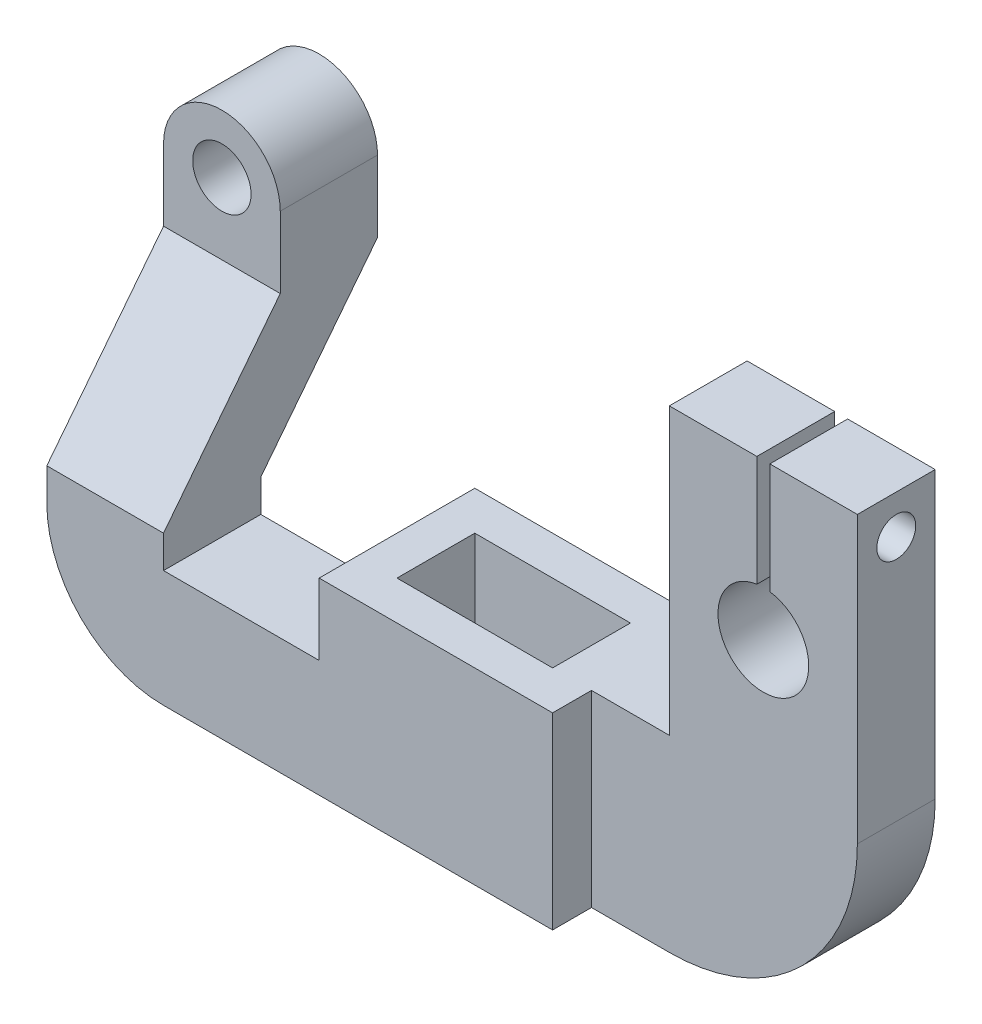
ISO-10303-21;
HEADER;
FILE_DESCRIPTION(('STEP AP214'),'2;1');
FILE_NAME('part.step','',(''),(''),'','','');
FILE_SCHEMA(('AUTOMOTIVE_DESIGN { 1 0 10303 214 1 1 1 1 }'));
ENDSEC;
DATA;
#1=APPLICATION_CONTEXT('core data for automotive mechanical design processes');
#2=APPLICATION_PROTOCOL_DEFINITION('international standard','automotive_design',2000,#1);
#3=PRODUCT_CONTEXT('',#1,'mechanical');
#4=PRODUCT('Part','Part','',(#3));
#5=PRODUCT_RELATED_PRODUCT_CATEGORY('part','',(#4));
#6=PRODUCT_DEFINITION_FORMATION('','',#4);
#7=PRODUCT_DEFINITION_CONTEXT('part definition',#1,'design');
#8=PRODUCT_DEFINITION('design','',#6,#7);
#9=PRODUCT_DEFINITION_SHAPE('','',#8);
#10=(LENGTH_UNIT() NAMED_UNIT(*) SI_UNIT(.MILLI.,.METRE.));
#11=(NAMED_UNIT(*) PLANE_ANGLE_UNIT() SI_UNIT($,.RADIAN.));
#12=(NAMED_UNIT(*) SI_UNIT($,.STERADIAN.) SOLID_ANGLE_UNIT());
#13=UNCERTAINTY_MEASURE_WITH_UNIT(LENGTH_MEASURE(1.E-05),#10,'distance_accuracy_value','');
#14=(GEOMETRIC_REPRESENTATION_CONTEXT(3) GLOBAL_UNCERTAINTY_ASSIGNED_CONTEXT((#13)) GLOBAL_UNIT_ASSIGNED_CONTEXT((#10,
#11,#12)) REPRESENTATION_CONTEXT('',''));
#15=CARTESIAN_POINT('',(0.,0.,0.));
#16=DIRECTION('',(0.,0.,1.));
#17=DIRECTION('',(1.,0.,0.));
#18=AXIS2_PLACEMENT_3D('',#15,#16,#17);
#19=CARTESIAN_POINT('',(48.,44.,6.));
#20=DIRECTION('',(0.,1.,0.));
#21=DIRECTION('',(0.,0.,1.));
#22=AXIS2_PLACEMENT_3D('',#19,#20,#21);
#23=PLANE('',#22);
#24=DIRECTION('',(0.,0.,1.));
#25=VECTOR('',#24,1.);
#26=CARTESIAN_POINT('',(63.5,44.,6.));
#27=LINE('',#26,#25);
#28=CARTESIAN_POINT('',(63.5,44.,6.));
#29=VERTEX_POINT('',#28);
#30=CARTESIAN_POINT('',(63.5,44.,18.));
#31=VERTEX_POINT('',#30);
#32=EDGE_CURVE('E285',#29,#31,#27,.T.);
#33=ORIENTED_EDGE('',*,*,#32,.T.);
#34=DIRECTION('',(-1.,0.,0.));
#35=VECTOR('',#34,1.);
#36=CARTESIAN_POINT('',(48.,44.,18.));
#37=LINE('',#36,#35);
#38=CARTESIAN_POINT('',(77.,44.,18.));
#39=VERTEX_POINT('',#38);
#40=EDGE_CURVE('E307',#39,#31,#37,.T.);
#41=ORIENTED_EDGE('',*,*,#40,.F.);
#42=DIRECTION('',(0.,0.,1.));
#43=VECTOR('',#42,1.);
#44=CARTESIAN_POINT('',(77.,44.,6.));
#45=LINE('',#44,#43);
#46=CARTESIAN_POINT('',(77.,44.,6.));
#47=VERTEX_POINT('',#46);
#48=EDGE_CURVE('E304',#47,#39,#45,.T.);
#49=ORIENTED_EDGE('',*,*,#48,.F.);
#50=DIRECTION('',(-1.,0.,0.));
#51=VECTOR('',#50,1.);
#52=CARTESIAN_POINT('',(48.,44.,6.));
#53=LINE('',#52,#51);
#54=EDGE_CURVE('E299',#47,#29,#53,.T.);
#55=ORIENTED_EDGE('',*,*,#54,.T.);
#56=EDGE_LOOP('',(#33,#41,#49,#55));
#57=FACE_BOUND('',#56,.T.);
#58=ADVANCED_FACE('F50',(#57),#23,.T.);
#59=CARTESIAN_POINT('',(0.,0.,24.));
#60=DIRECTION('',(0.,-1.,0.));
#61=DIRECTION('',(0.,0.,-1.));
#62=AXIS2_PLACEMENT_3D('',#59,#60,#61);
#63=PLANE('',#62);
#64=DIRECTION('',(1.,0.,0.));
#65=VECTOR('',#64,1.);
#66=CARTESIAN_POINT('',(6.,0.,18.));
#67=LINE('',#66,#65);
#68=CARTESIAN_POINT('',(6.,0.,18.));
#69=VERTEX_POINT('',#68);
#70=CARTESIAN_POINT('',(30.,0.,18.));
#71=VERTEX_POINT('',#70);
#72=EDGE_CURVE('E252',#69,#71,#67,.T.);
#73=ORIENTED_EDGE('',*,*,#72,.F.);
#74=DIRECTION('',(0.,0.,1.));
#75=VECTOR('',#74,1.);
#76=CARTESIAN_POINT('',(6.,0.,6.));
#77=LINE('',#76,#75);
#78=CARTESIAN_POINT('',(6.,0.,6.));
#79=VERTEX_POINT('',#78);
#80=EDGE_CURVE('E65',#79,#69,#77,.T.);
#81=ORIENTED_EDGE('',*,*,#80,.F.);
#82=DIRECTION('',(-1.,0.,0.));
#83=VECTOR('',#82,1.);
#84=CARTESIAN_POINT('',(6.,0.,6.));
#85=LINE('',#84,#83);
#86=CARTESIAN_POINT('',(30.,0.,6.));
#87=VERTEX_POINT('',#86);
#88=EDGE_CURVE('E260',#87,#79,#85,.T.);
#89=ORIENTED_EDGE('',*,*,#88,.F.);
#90=DIRECTION('',(0.,0.,-1.));
#91=VECTOR('',#90,1.);
#92=CARTESIAN_POINT('',(30.,0.,6.));
#93=LINE('',#92,#91);
#94=EDGE_CURVE('E245',#71,#87,#93,.T.);
#95=ORIENTED_EDGE('',*,*,#94,.F.);
#96=EDGE_LOOP('',(#73,#81,#89,#95));
#97=FACE_BOUND('',#96,.T.);
#98=DIRECTION('',(0.,0.,1.));
#99=VECTOR('',#98,1.);
#100=CARTESIAN_POINT('',(48.,0.,6.));
#101=LINE('',#100,#99);
#102=CARTESIAN_POINT('',(48.,0.,6.));
#103=VERTEX_POINT('',#102);
#104=CARTESIAN_POINT('',(48.,0.,18.));
#105=VERTEX_POINT('',#104);
#106=EDGE_CURVE('E313',#103,#105,#101,.T.);
#107=ORIENTED_EDGE('',*,*,#106,.F.);
#108=DIRECTION('',(-1.,0.,0.));
#109=VECTOR('',#108,1.);
#110=CARTESIAN_POINT('',(0.,0.,6.));
#111=LINE('',#110,#109);
#112=CARTESIAN_POINT('',(36.,0.,6.));
#113=VERTEX_POINT('',#112);
#114=EDGE_CURVE('E329',#103,#113,#111,.T.);
#115=ORIENTED_EDGE('',*,*,#114,.T.);
#116=DIRECTION('',(0.,0.,-1.));
#117=VECTOR('',#116,1.);
#118=CARTESIAN_POINT('',(36.,0.,24.));
#119=LINE('',#118,#117);
#120=CARTESIAN_POINT('',(36.,0.,0.));
#121=VERTEX_POINT('',#120);
#122=EDGE_CURVE('E457',#113,#121,#119,.T.);
#123=ORIENTED_EDGE('',*,*,#122,.T.);
#124=DIRECTION('',(-1.,0.,0.));
#125=VECTOR('',#124,1.);
#126=CARTESIAN_POINT('',(0.,0.,0.));
#127=LINE('',#126,#125);
#128=CARTESIAN_POINT('',(0.,0.,0.));
#129=VERTEX_POINT('',#128);
#130=EDGE_CURVE('E437',#121,#129,#127,.T.);
#131=ORIENTED_EDGE('',*,*,#130,.T.);
#132=DIRECTION('',(0.,0.,-1.));
#133=VECTOR('',#132,1.);
#134=CARTESIAN_POINT('',(0.,0.,24.));
#135=LINE('',#134,#133);
#136=CARTESIAN_POINT('',(0.,0.,24.));
#137=VERTEX_POINT('',#136);
#138=EDGE_CURVE('E444',#137,#129,#135,.T.);
#139=ORIENTED_EDGE('',*,*,#138,.F.);
#140=DIRECTION('',(-1.,0.,0.));
#141=VECTOR('',#140,1.);
#142=CARTESIAN_POINT('',(0.,0.,24.));
#143=LINE('',#142,#141);
#144=CARTESIAN_POINT('',(36.,0.,24.));
#145=VERTEX_POINT('',#144);
#146=EDGE_CURVE('E442',#145,#137,#143,.T.);
#147=ORIENTED_EDGE('',*,*,#146,.F.);
#148=CARTESIAN_POINT('',(36.,0.,18.));
#149=VERTEX_POINT('',#148);
#150=EDGE_CURVE('E459',#145,#149,#119,.T.);
#151=ORIENTED_EDGE('',*,*,#150,.T.);
#152=DIRECTION('',(1.,0.,0.));
#153=VECTOR('',#152,1.);
#154=CARTESIAN_POINT('',(0.,0.,18.));
#155=LINE('',#154,#153);
#156=EDGE_CURVE('E331',#149,#105,#155,.T.);
#157=ORIENTED_EDGE('',*,*,#156,.T.);
#158=EDGE_LOOP('',(#107,#115,#123,#131,#139,#147,#151,#157));
#159=FACE_BOUND('',#158,.T.);
#160=ADVANCED_FACE('F253',(#97,#159),#63,.F.);
#161=CARTESIAN_POINT('',(36.,0.,24.));
#162=DIRECTION('',(-1.,0.,0.));
#163=DIRECTION('',(0.,0.,1.));
#164=AXIS2_PLACEMENT_3D('',#161,#162,#163);
#165=PLANE('',#164);
#166=DIRECTION('',(0.,1.,0.));
#167=VECTOR('',#166,1.);
#168=CARTESIAN_POINT('',(36.,-29.,6.));
#169=LINE('',#168,#167);
#170=CARTESIAN_POINT('',(36.,-29.,6.));
#171=VERTEX_POINT('',#170);
#172=EDGE_CURVE('E336',#171,#113,#169,.T.);
#173=ORIENTED_EDGE('',*,*,#172,.F.);
#174=DIRECTION('',(0.,0.,-1.));
#175=VECTOR('',#174,1.);
#176=CARTESIAN_POINT('',(36.,-29.,24.));
#177=LINE('',#176,#175);
#178=CARTESIAN_POINT('',(36.,-29.,0.));
#179=VERTEX_POINT('',#178);
#180=EDGE_CURVE('E463',#171,#179,#177,.T.);
#181=ORIENTED_EDGE('',*,*,#180,.T.);
#182=DIRECTION('',(0.,1.,0.));
#183=VECTOR('',#182,1.);
#184=CARTESIAN_POINT('',(36.,0.,0.));
#185=LINE('',#184,#183);
#186=EDGE_CURVE('E454',#179,#121,#185,.T.);
#187=ORIENTED_EDGE('',*,*,#186,.T.);
#188=ORIENTED_EDGE('',*,*,#122,.F.);
#189=EDGE_LOOP('',(#173,#181,#187,#188));
#190=FACE_BOUND('',#189,.T.);
#191=ADVANCED_FACE('F499',(#190),#165,.F.);
#192=CARTESIAN_POINT('',(0.,-29.,24.));
#193=DIRECTION('',(1.,0.,0.));
#194=DIRECTION('',(0.,0.,-1.));
#195=AXIS2_PLACEMENT_3D('',#192,#193,#194);
#196=PLANE('',#195);
#197=DIRECTION('',(0.,0.,-1.));
#198=VECTOR('',#197,1.);
#199=CARTESIAN_POINT('',(0.,-29.,24.));
#200=LINE('',#199,#198);
#201=CARTESIAN_POINT('',(0.,-29.,9.));
#202=VERTEX_POINT('',#201);
#203=CARTESIAN_POINT('',(0.,-29.,0.));
#204=VERTEX_POINT('',#203);
#205=EDGE_CURVE('E462',#202,#204,#200,.T.);
#206=ORIENTED_EDGE('',*,*,#205,.F.);
#207=DIRECTION('',(0.,1.,0.));
#208=VECTOR('',#207,1.);
#209=CARTESIAN_POINT('',(0.,-11.,9.));
#210=LINE('',#209,#208);
#211=CARTESIAN_POINT('',(0.,-11.,9.));
#212=VERTEX_POINT('',#211);
#213=EDGE_CURVE('E387',#202,#212,#210,.T.);
#214=ORIENTED_EDGE('',*,*,#213,.T.);
#215=DIRECTION('',(0.,0.,1.));
#216=VECTOR('',#215,1.);
#217=CARTESIAN_POINT('',(0.,-11.,9.));
#218=LINE('',#217,#216);
#219=CARTESIAN_POINT('',(0.,-11.,24.));
#220=VERTEX_POINT('',#219);
#221=EDGE_CURVE('E412',#212,#220,#218,.T.);
#222=ORIENTED_EDGE('',*,*,#221,.T.);
#223=DIRECTION('',(0.,-1.,0.));
#224=VECTOR('',#223,1.);
#225=CARTESIAN_POINT('',(0.,-29.,24.));
#226=LINE('',#225,#224);
#227=EDGE_CURVE('E434',#137,#220,#226,.T.);
#228=ORIENTED_EDGE('',*,*,#227,.F.);
#229=ORIENTED_EDGE('',*,*,#138,.T.);
#230=DIRECTION('',(0.,-1.,0.));
#231=VECTOR('',#230,1.);
#232=CARTESIAN_POINT('',(0.,-29.,0.));
#233=LINE('',#232,#231);
#234=EDGE_CURVE('E426',#129,#204,#233,.T.);
#235=ORIENTED_EDGE('',*,*,#234,.T.);
#236=EDGE_LOOP('',(#206,#214,#222,#228,#229,#235));
#237=FACE_BOUND('',#236,.T.);
#238=ADVANCED_FACE('F47',(#237),#196,.F.);
#239=CARTESIAN_POINT('',(36.,-29.,24.));
#240=DIRECTION('',(0.,1.,0.));
#241=DIRECTION('',(0.,0.,1.));
#242=AXIS2_PLACEMENT_3D('',#239,#240,#241);
#243=PLANE('',#242);
#244=DIRECTION('',(-1.,0.,0.));
#245=VECTOR('',#244,1.);
#246=CARTESIAN_POINT('',(36.,-29.,6.));
#247=LINE('',#246,#245);
#248=CARTESIAN_POINT('',(30.,-29.,6.));
#249=VERTEX_POINT('',#248);
#250=CARTESIAN_POINT('',(6.,-29.,6.));
#251=VERTEX_POINT('',#250);
#252=EDGE_CURVE('E57',#249,#251,#247,.T.);
#253=ORIENTED_EDGE('',*,*,#252,.T.);
#254=DIRECTION('',(0.,0.,1.));
#255=VECTOR('',#254,1.);
#256=CARTESIAN_POINT('',(6.,-29.,24.));
#257=LINE('',#256,#255);
#258=CARTESIAN_POINT('',(6.,-29.,18.));
#259=VERTEX_POINT('',#258);
#260=EDGE_CURVE('E11',#251,#259,#257,.T.);
#261=ORIENTED_EDGE('',*,*,#260,.T.);
#262=DIRECTION('',(1.,0.,0.));
#263=VECTOR('',#262,1.);
#264=CARTESIAN_POINT('',(36.,-29.,18.));
#265=LINE('',#264,#263);
#266=CARTESIAN_POINT('',(30.,-29.,18.));
#267=VERTEX_POINT('',#266);
#268=EDGE_CURVE('E470',#259,#267,#265,.T.);
#269=ORIENTED_EDGE('',*,*,#268,.T.);
#270=DIRECTION('',(0.,0.,-1.));
#271=VECTOR('',#270,1.);
#272=CARTESIAN_POINT('',(30.,-29.,24.));
#273=LINE('',#272,#271);
#274=EDGE_CURVE('E244',#267,#249,#273,.T.);
#275=ORIENTED_EDGE('',*,*,#274,.T.);
#276=EDGE_LOOP('',(#253,#261,#269,#275));
#277=FACE_BOUND('',#276,.T.);
#278=DIRECTION('',(1.,0.,0.));
#279=VECTOR('',#278,1.);
#280=CARTESIAN_POINT('',(36.,-29.,0.));
#281=LINE('',#280,#279);
#282=EDGE_CURVE('E449',#204,#179,#281,.T.);
#283=ORIENTED_EDGE('',*,*,#282,.T.);
#284=ORIENTED_EDGE('',*,*,#180,.F.);
#285=DIRECTION('',(-1.,0.,0.));
#286=VECTOR('',#285,1.);
#287=CARTESIAN_POINT('',(0.,-29.,6.));
#288=LINE('',#287,#286);
#289=CARTESIAN_POINT('',(48.,-29.,6.));
#290=VERTEX_POINT('',#289);
#291=EDGE_CURVE('E335',#290,#171,#288,.T.);
#292=ORIENTED_EDGE('',*,*,#291,.F.);
#293=DIRECTION('',(0.,0.,-1.));
#294=VECTOR('',#293,1.);
#295=CARTESIAN_POINT('',(48.,-29.,0.));
#296=LINE('',#295,#294);
#297=CARTESIAN_POINT('',(48.,-29.,18.));
#298=VERTEX_POINT('',#297);
#299=EDGE_CURVE('E328',#298,#290,#296,.T.);
#300=ORIENTED_EDGE('',*,*,#299,.F.);
#301=DIRECTION('',(1.,0.,0.));
#302=VECTOR('',#301,1.);
#303=CARTESIAN_POINT('',(0.,-29.,18.));
#304=LINE('',#303,#302);
#305=CARTESIAN_POINT('',(36.,-29.,18.));
#306=VERTEX_POINT('',#305);
#307=EDGE_CURVE('E332',#306,#298,#304,.T.);
#308=ORIENTED_EDGE('',*,*,#307,.F.);
#309=CARTESIAN_POINT('',(36.,-29.,24.));
#310=VERTEX_POINT('',#309);
#311=EDGE_CURVE('E465',#310,#306,#177,.T.);
#312=ORIENTED_EDGE('',*,*,#311,.F.);
#313=DIRECTION('',(1.,0.,0.));
#314=VECTOR('',#313,1.);
#315=CARTESIAN_POINT('',(36.,-29.,24.));
#316=LINE('',#315,#314);
#317=CARTESIAN_POINT('',(-24.,-29.,24.));
#318=VERTEX_POINT('',#317);
#319=EDGE_CURVE('E438',#318,#310,#316,.T.);
#320=ORIENTED_EDGE('',*,*,#319,.F.);
#321=DIRECTION('',(0.,0.,1.));
#322=VECTOR('',#321,1.);
#323=CARTESIAN_POINT('',(-24.,-29.,9.));
#324=LINE('',#323,#322);
#325=CARTESIAN_POINT('',(-24.,-29.,9.));
#326=VERTEX_POINT('',#325);
#327=EDGE_CURVE('E424',#326,#318,#324,.T.);
#328=ORIENTED_EDGE('',*,*,#327,.F.);
#329=DIRECTION('',(1.,0.,0.));
#330=VECTOR('',#329,1.);
#331=CARTESIAN_POINT('',(0.,-29.,9.));
#332=LINE('',#331,#330);
#333=EDGE_CURVE('E408',#326,#202,#332,.T.);
#334=ORIENTED_EDGE('',*,*,#333,.T.);
#335=ORIENTED_EDGE('',*,*,#205,.T.);
#336=EDGE_LOOP('',(#283,#284,#292,#300,#308,#312,#320,#328,#334,#335));
#337=FACE_BOUND('',#336,.T.);
#338=ADVANCED_FACE('F471',(#277,#337),#243,.F.);
#339=ORIENTED_EDGE('',*,*,#311,.T.);
#340=DIRECTION('',(0.,1.,0.));
#341=VECTOR('',#340,1.);
#342=CARTESIAN_POINT('',(36.,-29.,18.));
#343=LINE('',#342,#341);
#344=EDGE_CURVE('E344',#306,#149,#343,.T.);
#345=ORIENTED_EDGE('',*,*,#344,.T.);
#346=ORIENTED_EDGE('',*,*,#150,.F.);
#347=DIRECTION('',(0.,1.,0.));
#348=VECTOR('',#347,1.);
#349=CARTESIAN_POINT('',(36.,0.,24.));
#350=LINE('',#349,#348);
#351=EDGE_CURVE('E441',#310,#145,#350,.T.);
#352=ORIENTED_EDGE('',*,*,#351,.F.);
#353=EDGE_LOOP('',(#339,#345,#346,#352));
#354=FACE_BOUND('',#353,.T.);
#355=ADVANCED_FACE('F551',(#354),#165,.F.);
#356=CARTESIAN_POINT('',(0.,0.,24.));
#357=DIRECTION('',(0.,0.,-1.));
#358=DIRECTION('',(-1.,0.,0.));
#359=AXIS2_PLACEMENT_3D('',#356,#357,#358);
#360=PLANE('',#359);
#361=ORIENTED_EDGE('',*,*,#227,.T.);
#362=DIRECTION('',(-1.,0.,0.));
#363=VECTOR('',#362,1.);
#364=CARTESIAN_POINT('',(-24.,-11.,24.));
#365=LINE('',#364,#363);
#366=CARTESIAN_POINT('',(-24.,-11.,24.));
#367=VERTEX_POINT('',#366);
#368=EDGE_CURVE('E390',#220,#367,#365,.T.);
#369=ORIENTED_EDGE('',*,*,#368,.T.);
#370=DIRECTION('',(0.,1.,0.));
#371=VECTOR('',#370,1.);
#372=CARTESIAN_POINT('',(-24.,-11.,24.));
#373=LINE('',#372,#371);
#374=CARTESIAN_POINT('',(-24.,-6.,24.));
#375=VERTEX_POINT('',#374);
#376=EDGE_CURVE('E415',#367,#375,#373,.T.);
#377=ORIENTED_EDGE('',*,*,#376,.T.);
#378=DIRECTION('',(-1.,0.,0.));
#379=VECTOR('',#378,1.);
#380=CARTESIAN_POINT('',(-41.2916164657906,-6.,24.));
#381=LINE('',#380,#379);
#382=CARTESIAN_POINT('',(-42.,-6.,24.));
#383=VERTEX_POINT('',#382);
#384=EDGE_CURVE('E420',#375,#383,#381,.T.);
#385=ORIENTED_EDGE('',*,*,#384,.T.);
#386=DIRECTION('',(0.,-1.,0.));
#387=VECTOR('',#386,1.);
#388=CARTESIAN_POINT('',(-42.,-6.,24.));
#389=LINE('',#388,#387);
#390=CARTESIAN_POINT('',(-42.,-11.,24.));
#391=VERTEX_POINT('',#390);
#392=EDGE_CURVE('E417',#383,#391,#389,.T.);
#393=ORIENTED_EDGE('',*,*,#392,.T.);
#394=CARTESIAN_POINT('',(-24.,-11.,24.));
#395=DIRECTION('',(0.,0.,1.));
#396=DIRECTION('',(1.,0.,0.));
#397=AXIS2_PLACEMENT_3D('',#394,#395,#396);
#398=CIRCLE('',#397,18.);
#399=EDGE_CURVE('E393',#391,#318,#398,.T.);
#400=ORIENTED_EDGE('',*,*,#399,.T.);
#401=ORIENTED_EDGE('',*,*,#319,.T.);
#402=ORIENTED_EDGE('',*,*,#351,.T.);
#403=ORIENTED_EDGE('',*,*,#146,.T.);
#404=EDGE_LOOP('',(#361,#369,#377,#385,#393,#400,#401,#402,#403));
#405=FACE_BOUND('',#404,.T.);
#406=ADVANCED_FACE('F559',(#405),#360,.F.);
#407=CARTESIAN_POINT('',(0.,0.,0.));
#408=DIRECTION('',(0.,0.,-1.));
#409=DIRECTION('',(-1.,0.,0.));
#410=AXIS2_PLACEMENT_3D('',#407,#408,#409);
#411=PLANE('',#410);
#412=ORIENTED_EDGE('',*,*,#234,.F.);
#413=ORIENTED_EDGE('',*,*,#130,.F.);
#414=ORIENTED_EDGE('',*,*,#186,.F.);
#415=ORIENTED_EDGE('',*,*,#282,.F.);
#416=EDGE_LOOP('',(#412,#413,#414,#415));
#417=FACE_BOUND('',#416,.T.);
#418=ADVANCED_FACE('F573',(#417),#411,.T.);
#419=CARTESIAN_POINT('',(-24.,-11.,9.));
#420=DIRECTION('',(0.,0.,1.));
#421=DIRECTION('',(1.,0.,0.));
#422=AXIS2_PLACEMENT_3D('',#419,#420,#421);
#423=CYLINDRICAL_SURFACE('',#422,18.);
#424=ORIENTED_EDGE('',*,*,#399,.F.);
#425=DIRECTION('',(0.,0.,1.));
#426=VECTOR('',#425,1.);
#427=CARTESIAN_POINT('',(-42.,-11.,9.));
#428=LINE('',#427,#426);
#429=CARTESIAN_POINT('',(-42.,-11.,9.));
#430=VERTEX_POINT('',#429);
#431=EDGE_CURVE('E429',#430,#391,#428,.T.);
#432=ORIENTED_EDGE('',*,*,#431,.F.);
#433=CARTESIAN_POINT('',(-24.,-11.,9.));
#434=DIRECTION('',(0.,0.,1.));
#435=DIRECTION('',(1.,0.,0.));
#436=AXIS2_PLACEMENT_3D('',#433,#434,#435);
#437=CIRCLE('',#436,18.);
#438=EDGE_CURVE('E409',#430,#326,#437,.T.);
#439=ORIENTED_EDGE('',*,*,#438,.T.);
#440=ORIENTED_EDGE('',*,*,#327,.T.);
#441=EDGE_LOOP('',(#424,#432,#439,#440));
#442=FACE_BOUND('',#441,.T.);
#443=ADVANCED_FACE('F565',(#442),#423,.T.);
#444=CARTESIAN_POINT('',(-42.,-6.,9.));
#445=DIRECTION('',(-1.,0.,0.));
#446=DIRECTION('',(0.,0.,1.));
#447=AXIS2_PLACEMENT_3D('',#444,#445,#446);
#448=PLANE('',#447);
#449=ORIENTED_EDGE('',*,*,#392,.F.);
#450=DIRECTION('',(0.,0.787505001007586,-0.616308261658111));
#451=VECTOR('',#450,1.);
#452=CARTESIAN_POINT('',(-42.,17.,6.));
#453=LINE('',#452,#451);
#454=CARTESIAN_POINT('',(-42.,17.,6.));
#455=VERTEX_POINT('',#454);
#456=EDGE_CURVE('E366',#383,#455,#453,.T.);
#457=ORIENTED_EDGE('',*,*,#456,.T.);
#458=DIRECTION('',(0.,1.,0.));
#459=VECTOR('',#458,1.);
#460=CARTESIAN_POINT('',(-42.,28.,6.));
#461=LINE('',#460,#459);
#462=CARTESIAN_POINT('',(-42.,28.,6.));
#463=VERTEX_POINT('',#462);
#464=EDGE_CURVE('E352',#455,#463,#461,.T.);
#465=ORIENTED_EDGE('',*,*,#464,.T.);
#466=DIRECTION('',(0.,0.,-1.));
#467=VECTOR('',#466,1.);
#468=CARTESIAN_POINT('',(-42.,28.,-9.));
#469=LINE('',#468,#467);
#470=CARTESIAN_POINT('',(-42.,28.,-9.));
#471=VERTEX_POINT('',#470);
#472=EDGE_CURVE('E367',#463,#471,#469,.T.);
#473=ORIENTED_EDGE('',*,*,#472,.T.);
#474=DIRECTION('',(0.,-1.,0.));
#475=VECTOR('',#474,1.);
#476=CARTESIAN_POINT('',(-42.,17.,-9.));
#477=LINE('',#476,#475);
#478=CARTESIAN_POINT('',(-42.,17.,-9.));
#479=VERTEX_POINT('',#478);
#480=EDGE_CURVE('E363',#471,#479,#477,.T.);
#481=ORIENTED_EDGE('',*,*,#480,.T.);
#482=DIRECTION('',(0.,-0.787505001007586,0.616308261658111));
#483=VECTOR('',#482,1.);
#484=CARTESIAN_POINT('',(-42.,17.,-9.));
#485=LINE('',#484,#483);
#486=CARTESIAN_POINT('',(-42.,-6.,9.));
#487=VERTEX_POINT('',#486);
#488=EDGE_CURVE('E380',#479,#487,#485,.T.);
#489=ORIENTED_EDGE('',*,*,#488,.T.);
#490=DIRECTION('',(0.,-1.,0.));
#491=VECTOR('',#490,1.);
#492=CARTESIAN_POINT('',(-42.,-6.,9.));
#493=LINE('',#492,#491);
#494=EDGE_CURVE('E401',#487,#430,#493,.T.);
#495=ORIENTED_EDGE('',*,*,#494,.T.);
#496=ORIENTED_EDGE('',*,*,#431,.T.);
#497=EDGE_LOOP('',(#449,#457,#465,#473,#481,#489,#495,#496));
#498=FACE_BOUND('',#497,.T.);
#499=ADVANCED_FACE('F841',(#498),#448,.T.);
#500=CARTESIAN_POINT('',(-24.,-11.,9.));
#501=DIRECTION('',(1.,0.,0.));
#502=DIRECTION('',(0.,0.,-1.));
#503=AXIS2_PLACEMENT_3D('',#500,#501,#502);
#504=PLANE('',#503);
#505=ORIENTED_EDGE('',*,*,#376,.F.);
#506=DIRECTION('',(0.,0.,1.));
#507=VECTOR('',#506,1.);
#508=CARTESIAN_POINT('',(-24.,-11.,9.));
#509=LINE('',#508,#507);
#510=CARTESIAN_POINT('',(-24.,-11.,9.));
#511=VERTEX_POINT('',#510);
#512=EDGE_CURVE('E431',#511,#367,#509,.T.);
#513=ORIENTED_EDGE('',*,*,#512,.F.);
#514=DIRECTION('',(0.,1.,0.));
#515=VECTOR('',#514,1.);
#516=CARTESIAN_POINT('',(-24.,-11.,9.));
#517=LINE('',#516,#515);
#518=CARTESIAN_POINT('',(-24.,-6.,9.));
#519=VERTEX_POINT('',#518);
#520=EDGE_CURVE('E400',#511,#519,#517,.T.);
#521=ORIENTED_EDGE('',*,*,#520,.T.);
#522=DIRECTION('',(0.,-0.787505001007586,0.616308261658111));
#523=VECTOR('',#522,1.);
#524=CARTESIAN_POINT('',(-24.,17.,-9.));
#525=LINE('',#524,#523);
#526=CARTESIAN_POINT('',(-24.,17.,-9.));
#527=VERTEX_POINT('',#526);
#528=EDGE_CURVE('E376',#527,#519,#525,.T.);
#529=ORIENTED_EDGE('',*,*,#528,.F.);
#530=DIRECTION('',(0.,-1.,0.));
#531=VECTOR('',#530,1.);
#532=CARTESIAN_POINT('',(-24.,17.,-9.));
#533=LINE('',#532,#531);
#534=CARTESIAN_POINT('',(-24.,28.,-9.));
#535=VERTEX_POINT('',#534);
#536=EDGE_CURVE('E361',#535,#527,#533,.T.);
#537=ORIENTED_EDGE('',*,*,#536,.F.);
#538=DIRECTION('',(0.,0.,-1.));
#539=VECTOR('',#538,1.);
#540=CARTESIAN_POINT('',(-24.,28.,-9.));
#541=LINE('',#540,#539);
#542=CARTESIAN_POINT('',(-24.,28.,6.));
#543=VERTEX_POINT('',#542);
#544=EDGE_CURVE('E359',#543,#535,#541,.T.);
#545=ORIENTED_EDGE('',*,*,#544,.F.);
#546=DIRECTION('',(0.,1.,0.));
#547=VECTOR('',#546,1.);
#548=CARTESIAN_POINT('',(-24.,28.,6.));
#549=LINE('',#548,#547);
#550=CARTESIAN_POINT('',(-24.,17.,6.));
#551=VERTEX_POINT('',#550);
#552=EDGE_CURVE('E357',#551,#543,#549,.T.);
#553=ORIENTED_EDGE('',*,*,#552,.F.);
#554=DIRECTION('',(0.,0.787505001007586,-0.616308261658111));
#555=VECTOR('',#554,1.);
#556=CARTESIAN_POINT('',(-24.,17.,6.));
#557=LINE('',#556,#555);
#558=EDGE_CURVE('E372',#375,#551,#557,.T.);
#559=ORIENTED_EDGE('',*,*,#558,.F.);
#560=EDGE_LOOP('',(#505,#513,#521,#529,#537,#545,#553,#559));
#561=FACE_BOUND('',#560,.T.);
#562=ADVANCED_FACE('F835',(#561),#504,.T.);
#563=CARTESIAN_POINT('',(-24.,-11.,9.));
#564=DIRECTION('',(0.,1.,0.));
#565=DIRECTION('',(-1.,0.,0.));
#566=AXIS2_PLACEMENT_3D('',#563,#564,#565);
#567=PLANE('',#566);
#568=ORIENTED_EDGE('',*,*,#368,.F.);
#569=ORIENTED_EDGE('',*,*,#221,.F.);
#570=DIRECTION('',(-1.,0.,0.));
#571=VECTOR('',#570,1.);
#572=CARTESIAN_POINT('',(-24.,-11.,9.));
#573=LINE('',#572,#571);
#574=EDGE_CURVE('E394',#212,#511,#573,.T.);
#575=ORIENTED_EDGE('',*,*,#574,.T.);
#576=ORIENTED_EDGE('',*,*,#512,.T.);
#577=EDGE_LOOP('',(#568,#569,#575,#576));
#578=FACE_BOUND('',#577,.T.);
#579=ADVANCED_FACE('F825',(#578),#567,.T.);
#580=CARTESIAN_POINT('',(-24.,-11.,9.));
#581=DIRECTION('',(0.,0.,1.));
#582=DIRECTION('',(1.,0.,0.));
#583=AXIS2_PLACEMENT_3D('',#580,#581,#582);
#584=PLANE('',#583);
#585=ORIENTED_EDGE('',*,*,#213,.F.);
#586=ORIENTED_EDGE('',*,*,#333,.F.);
#587=ORIENTED_EDGE('',*,*,#438,.F.);
#588=ORIENTED_EDGE('',*,*,#494,.F.);
#589=DIRECTION('',(-1.,0.,0.));
#590=VECTOR('',#589,1.);
#591=CARTESIAN_POINT('',(-24.,-6.,9.));
#592=LINE('',#591,#590);
#593=EDGE_CURVE('E397',#519,#487,#592,.T.);
#594=ORIENTED_EDGE('',*,*,#593,.F.);
#595=ORIENTED_EDGE('',*,*,#520,.F.);
#596=ORIENTED_EDGE('',*,*,#574,.F.);
#597=EDGE_LOOP('',(#585,#586,#587,#588,#594,#595,#596));
#598=FACE_BOUND('',#597,.T.);
#599=ADVANCED_FACE('F566',(#598),#584,.F.);
#600=CARTESIAN_POINT('',(-24.,17.,-9.));
#601=DIRECTION('',(0.,-0.616308261658111,-0.787505001007586));
#602=DIRECTION('',(0.,0.787505001007586,-0.616308261658111));
#603=AXIS2_PLACEMENT_3D('',#600,#601,#602);
#604=PLANE('',#603);
#605=ORIENTED_EDGE('',*,*,#488,.F.);
#606=DIRECTION('',(-1.,0.,0.));
#607=VECTOR('',#606,1.);
#608=CARTESIAN_POINT('',(-24.,17.,-9.));
#609=LINE('',#608,#607);
#610=EDGE_CURVE('E383',#527,#479,#609,.T.);
#611=ORIENTED_EDGE('',*,*,#610,.F.);
#612=ORIENTED_EDGE('',*,*,#528,.T.);
#613=ORIENTED_EDGE('',*,*,#593,.T.);
#614=EDGE_LOOP('',(#605,#611,#612,#613));
#615=FACE_BOUND('',#614,.T.);
#616=ADVANCED_FACE('F801',(#615),#604,.T.);
#617=CARTESIAN_POINT('',(-24.,17.,6.));
#618=DIRECTION('',(0.,0.616308261658111,0.787505001007586));
#619=DIRECTION('',(0.,-0.787505001007586,0.616308261658111));
#620=AXIS2_PLACEMENT_3D('',#617,#618,#619);
#621=PLANE('',#620);
#622=ORIENTED_EDGE('',*,*,#456,.F.);
#623=ORIENTED_EDGE('',*,*,#384,.F.);
#624=ORIENTED_EDGE('',*,*,#558,.T.);
#625=DIRECTION('',(-1.,0.,0.));
#626=VECTOR('',#625,1.);
#627=CARTESIAN_POINT('',(-24.,17.,6.));
#628=LINE('',#627,#626);
#629=EDGE_CURVE('E379',#551,#455,#628,.T.);
#630=ORIENTED_EDGE('',*,*,#629,.T.);
#631=EDGE_LOOP('',(#622,#623,#624,#630));
#632=FACE_BOUND('',#631,.T.);
#633=ADVANCED_FACE('F792',(#632),#621,.T.);
#634=CARTESIAN_POINT('',(-24.,17.,-9.));
#635=DIRECTION('',(0.,0.,-1.));
#636=DIRECTION('',(-1.,0.,0.));
#637=AXIS2_PLACEMENT_3D('',#634,#635,#636);
#638=PLANE('',#637);
#639=CARTESIAN_POINT('',(-33.,28.,-9.));
#640=DIRECTION('',(0.,0.,1.));
#641=DIRECTION('',(1.,0.,0.));
#642=AXIS2_PLACEMENT_3D('',#639,#640,#641);
#643=CIRCLE('',#642,4.5);
#644=CARTESIAN_POINT('',(-28.5,28.,-9.));
#645=VERTEX_POINT('',#644);
#646=EDGE_CURVE('E347',#645,#645,#643,.T.);
#647=ORIENTED_EDGE('',*,*,#646,.T.);
#648=EDGE_LOOP('',(#647));
#649=FACE_BOUND('',#648,.T.);
#650=ORIENTED_EDGE('',*,*,#480,.F.);
#651=CARTESIAN_POINT('',(-33.,28.,-9.));
#652=DIRECTION('',(0.,0.,1.));
#653=DIRECTION('',(1.,0.,0.));
#654=AXIS2_PLACEMENT_3D('',#651,#652,#653);
#655=CIRCLE('',#654,9.);
#656=EDGE_CURVE('E351',#535,#471,#655,.T.);
#657=ORIENTED_EDGE('',*,*,#656,.F.);
#658=ORIENTED_EDGE('',*,*,#536,.T.);
#659=ORIENTED_EDGE('',*,*,#610,.T.);
#660=EDGE_LOOP('',(#650,#657,#658,#659));
#661=FACE_BOUND('',#660,.T.);
#662=ADVANCED_FACE('F781',(#649,#661),#638,.T.);
#663=CARTESIAN_POINT('',(-24.,28.,6.));
#664=DIRECTION('',(0.,0.,1.));
#665=DIRECTION('',(1.,0.,0.));
#666=AXIS2_PLACEMENT_3D('',#663,#664,#665);
#667=PLANE('',#666);
#668=CARTESIAN_POINT('',(-33.,28.,6.));
#669=DIRECTION('',(0.,0.,1.));
#670=DIRECTION('',(1.,0.,0.));
#671=AXIS2_PLACEMENT_3D('',#668,#669,#670);
#672=CIRCLE('',#671,4.5);
#673=CARTESIAN_POINT('',(-28.5,28.,6.));
#674=VERTEX_POINT('',#673);
#675=EDGE_CURVE('E343',#674,#674,#672,.T.);
#676=ORIENTED_EDGE('',*,*,#675,.F.);
#677=EDGE_LOOP('',(#676));
#678=FACE_BOUND('',#677,.T.);
#679=ORIENTED_EDGE('',*,*,#464,.F.);
#680=ORIENTED_EDGE('',*,*,#629,.F.);
#681=ORIENTED_EDGE('',*,*,#552,.T.);
#682=CARTESIAN_POINT('',(-33.,28.,6.));
#683=DIRECTION('',(0.,0.,1.));
#684=DIRECTION('',(1.,0.,0.));
#685=AXIS2_PLACEMENT_3D('',#682,#683,#684);
#686=CIRCLE('',#685,9.);
#687=EDGE_CURVE('E350',#543,#463,#686,.T.);
#688=ORIENTED_EDGE('',*,*,#687,.T.);
#689=EDGE_LOOP('',(#679,#680,#681,#688));
#690=FACE_BOUND('',#689,.T.);
#691=ADVANCED_FACE('F769',(#678,#690),#667,.T.);
#692=CARTESIAN_POINT('',(-33.,28.,-9.));
#693=DIRECTION('',(0.,0.,1.));
#694=DIRECTION('',(1.,0.,0.));
#695=AXIS2_PLACEMENT_3D('',#692,#693,#694);
#696=CYLINDRICAL_SURFACE('',#695,9.);
#697=ORIENTED_EDGE('',*,*,#687,.F.);
#698=ORIENTED_EDGE('',*,*,#544,.T.);
#699=ORIENTED_EDGE('',*,*,#656,.T.);
#700=ORIENTED_EDGE('',*,*,#472,.F.);
#701=EDGE_LOOP('',(#697,#698,#699,#700));
#702=FACE_BOUND('',#701,.T.);
#703=ADVANCED_FACE('F761',(#702),#696,.T.);
#704=CARTESIAN_POINT('',(-33.,28.,-9.));
#705=DIRECTION('',(0.,0.,1.));
#706=DIRECTION('',(1.,0.,0.));
#707=AXIS2_PLACEMENT_3D('',#704,#705,#706);
#708=CYLINDRICAL_SURFACE('',#707,4.5);
#709=ORIENTED_EDGE('',*,*,#646,.F.);
#710=EDGE_LOOP('',(#709));
#711=FACE_BOUND('',#710,.T.);
#712=ORIENTED_EDGE('',*,*,#675,.T.);
#713=EDGE_LOOP('',(#712));
#714=FACE_BOUND('',#713,.T.);
#715=ADVANCED_FACE('F734',(#711,#714),#708,.F.);
#716=CARTESIAN_POINT('',(0.,-29.,18.));
#717=DIRECTION('',(0.,0.,1.));
#718=DIRECTION('',(1.,0.,0.));
#719=AXIS2_PLACEMENT_3D('',#716,#717,#718);
#720=PLANE('',#719);
#721=DIRECTION('',(0.,1.,0.));
#722=VECTOR('',#721,1.);
#723=CARTESIAN_POINT('',(63.5,44.,18.));
#724=LINE('',#723,#722);
#725=CARTESIAN_POINT('',(63.5,26.9282032302755,18.));
#726=VERTEX_POINT('',#725);
#727=EDGE_CURVE('E275',#726,#31,#724,.T.);
#728=ORIENTED_EDGE('',*,*,#727,.F.);
#729=CARTESIAN_POINT('',(62.5,20.,18.));
#730=DIRECTION('',(0.,0.,1.));
#731=DIRECTION('',(1.,0.,0.));
#732=AXIS2_PLACEMENT_3D('',#729,#730,#731);
#733=CIRCLE('',#732,7.);
#734=CARTESIAN_POINT('',(61.5,26.9282032302755,18.));
#735=VERTEX_POINT('',#734);
#736=EDGE_CURVE('E281',#735,#726,#733,.T.);
#737=ORIENTED_EDGE('',*,*,#736,.F.);
#738=DIRECTION('',(0.,-1.,0.));
#739=VECTOR('',#738,1.);
#740=CARTESIAN_POINT('',(61.5,44.,18.));
#741=LINE('',#740,#739);
#742=CARTESIAN_POINT('',(61.5,44.,18.));
#743=VERTEX_POINT('',#742);
#744=EDGE_CURVE('E265',#743,#735,#741,.T.);
#745=ORIENTED_EDGE('',*,*,#744,.F.);
#746=CARTESIAN_POINT('',(48.,44.,18.));
#747=VERTEX_POINT('',#746);
#748=EDGE_CURVE('E308',#743,#747,#37,.T.);
#749=ORIENTED_EDGE('',*,*,#748,.T.);
#750=DIRECTION('',(0.,-1.,0.));
#751=VECTOR('',#750,1.);
#752=CARTESIAN_POINT('',(48.,0.,18.));
#753=LINE('',#752,#751);
#754=EDGE_CURVE('E296',#747,#105,#753,.T.);
#755=ORIENTED_EDGE('',*,*,#754,.T.);
#756=ORIENTED_EDGE('',*,*,#156,.F.);
#757=ORIENTED_EDGE('',*,*,#344,.F.);
#758=ORIENTED_EDGE('',*,*,#307,.T.);
#759=CARTESIAN_POINT('',(48.,0.,18.));
#760=DIRECTION('',(0.,0.,1.));
#761=DIRECTION('',(1.,0.,0.));
#762=AXIS2_PLACEMENT_3D('',#759,#760,#761);
#763=CIRCLE('',#762,29.);
#764=CARTESIAN_POINT('',(77.,0.,18.));
#765=VERTEX_POINT('',#764);
#766=EDGE_CURVE('E320',#298,#765,#763,.T.);
#767=ORIENTED_EDGE('',*,*,#766,.T.);
#768=DIRECTION('',(0.,1.,0.));
#769=VECTOR('',#768,1.);
#770=CARTESIAN_POINT('',(77.,44.,18.));
#771=LINE('',#770,#769);
#772=EDGE_CURVE('E286',#765,#39,#771,.T.);
#773=ORIENTED_EDGE('',*,*,#772,.T.);
#774=ORIENTED_EDGE('',*,*,#40,.T.);
#775=EDGE_LOOP('',(#728,#737,#745,#749,#755,#756,#757,#758,#767,#773,#774));
#776=FACE_BOUND('',#775,.T.);
#777=ADVANCED_FACE('F535',(#776),#720,.T.);
#778=CARTESIAN_POINT('',(0.,-29.,6.));
#779=DIRECTION('',(0.,0.,-1.));
#780=DIRECTION('',(-1.,0.,0.));
#781=AXIS2_PLACEMENT_3D('',#778,#779,#780);
#782=PLANE('',#781);
#783=DIRECTION('',(0.,1.,0.));
#784=VECTOR('',#783,1.);
#785=CARTESIAN_POINT('',(63.5,44.,6.));
#786=LINE('',#785,#784);
#787=CARTESIAN_POINT('',(63.5,26.9282032302755,6.));
#788=VERTEX_POINT('',#787);
#789=EDGE_CURVE('E273',#788,#29,#786,.T.);
#790=ORIENTED_EDGE('',*,*,#789,.T.);
#791=ORIENTED_EDGE('',*,*,#54,.F.);
#792=DIRECTION('',(0.,1.,0.));
#793=VECTOR('',#792,1.);
#794=CARTESIAN_POINT('',(77.,44.,6.));
#795=LINE('',#794,#793);
#796=CARTESIAN_POINT('',(77.,0.,6.));
#797=VERTEX_POINT('',#796);
#798=EDGE_CURVE('E295',#797,#47,#795,.T.);
#799=ORIENTED_EDGE('',*,*,#798,.F.);
#800=CARTESIAN_POINT('',(48.,0.,6.));
#801=DIRECTION('',(0.,0.,1.));
#802=DIRECTION('',(1.,0.,0.));
#803=AXIS2_PLACEMENT_3D('',#800,#801,#802);
#804=CIRCLE('',#803,29.);
#805=EDGE_CURVE('E321',#290,#797,#804,.T.);
#806=ORIENTED_EDGE('',*,*,#805,.F.);
#807=ORIENTED_EDGE('',*,*,#291,.T.);
#808=ORIENTED_EDGE('',*,*,#172,.T.);
#809=ORIENTED_EDGE('',*,*,#114,.F.);
#810=DIRECTION('',(0.,-1.,0.));
#811=VECTOR('',#810,1.);
#812=CARTESIAN_POINT('',(48.,0.,6.));
#813=LINE('',#812,#811);
#814=CARTESIAN_POINT('',(48.,44.,6.));
#815=VERTEX_POINT('',#814);
#816=EDGE_CURVE('E305',#815,#103,#813,.T.);
#817=ORIENTED_EDGE('',*,*,#816,.F.);
#818=CARTESIAN_POINT('',(61.5,44.,6.));
#819=VERTEX_POINT('',#818);
#820=EDGE_CURVE('E300',#819,#815,#53,.T.);
#821=ORIENTED_EDGE('',*,*,#820,.F.);
#822=DIRECTION('',(0.,-1.,0.));
#823=VECTOR('',#822,1.);
#824=CARTESIAN_POINT('',(61.5,44.,6.));
#825=LINE('',#824,#823);
#826=CARTESIAN_POINT('',(61.5,26.9282032302755,6.));
#827=VERTEX_POINT('',#826);
#828=EDGE_CURVE('E266',#819,#827,#825,.T.);
#829=ORIENTED_EDGE('',*,*,#828,.T.);
#830=CARTESIAN_POINT('',(62.5,20.,6.));
#831=DIRECTION('',(0.,0.,1.));
#832=DIRECTION('',(1.,0.,0.));
#833=AXIS2_PLACEMENT_3D('',#830,#831,#832);
#834=CIRCLE('',#833,7.);
#835=EDGE_CURVE('E272',#827,#788,#834,.T.);
#836=ORIENTED_EDGE('',*,*,#835,.T.);
#837=EDGE_LOOP('',(#790,#791,#799,#806,#807,#808,#809,#817,#821,#829,#836));
#838=FACE_BOUND('',#837,.T.);
#839=ADVANCED_FACE('F528',(#838),#782,.T.);
#840=CARTESIAN_POINT('',(48.,0.,6.));
#841=DIRECTION('',(0.,0.,1.));
#842=DIRECTION('',(1.,0.,0.));
#843=AXIS2_PLACEMENT_3D('',#840,#841,#842);
#844=CYLINDRICAL_SURFACE('',#843,29.);
#845=ORIENTED_EDGE('',*,*,#766,.F.);
#846=ORIENTED_EDGE('',*,*,#299,.T.);
#847=ORIENTED_EDGE('',*,*,#805,.T.);
#848=DIRECTION('',(0.,0.,1.));
#849=VECTOR('',#848,1.);
#850=CARTESIAN_POINT('',(77.,0.,6.));
#851=LINE('',#850,#849);
#852=EDGE_CURVE('E323',#797,#765,#851,.T.);
#853=ORIENTED_EDGE('',*,*,#852,.T.);
#854=EDGE_LOOP('',(#845,#846,#847,#853));
#855=FACE_BOUND('',#854,.T.);
#856=ADVANCED_FACE('F519',(#855),#844,.T.);
#857=CARTESIAN_POINT('',(48.,0.,6.));
#858=DIRECTION('',(-1.,0.,0.));
#859=DIRECTION('',(0.,0.,1.));
#860=AXIS2_PLACEMENT_3D('',#857,#858,#859);
#861=PLANE('',#860);
#862=CARTESIAN_POINT('',(48.,38.,12.));
#863=DIRECTION('',(-1.,0.,0.));
#864=DIRECTION('',(0.,0.,1.));
#865=AXIS2_PLACEMENT_3D('',#862,#863,#864);
#866=CIRCLE('',#865,3.);
#867=CARTESIAN_POINT('',(48.,38.,15.));
#868=VERTEX_POINT('',#867);
#869=EDGE_CURVE('E1034',#868,#868,#866,.T.);
#870=ORIENTED_EDGE('',*,*,#869,.F.);
#871=EDGE_LOOP('',(#870));
#872=FACE_BOUND('',#871,.T.);
#873=ORIENTED_EDGE('',*,*,#754,.F.);
#874=DIRECTION('',(0.,0.,1.));
#875=VECTOR('',#874,1.);
#876=CARTESIAN_POINT('',(48.,44.,6.));
#877=LINE('',#876,#875);
#878=EDGE_CURVE('E319',#815,#747,#877,.T.);
#879=ORIENTED_EDGE('',*,*,#878,.F.);
#880=ORIENTED_EDGE('',*,*,#816,.T.);
#881=ORIENTED_EDGE('',*,*,#106,.T.);
#882=EDGE_LOOP('',(#873,#879,#880,#881));
#883=FACE_BOUND('',#882,.T.);
#884=ADVANCED_FACE('F506',(#872,#883),#861,.T.);
#885=DIRECTION('',(0.,0.,1.));
#886=VECTOR('',#885,1.);
#887=CARTESIAN_POINT('',(61.5,44.,6.));
#888=LINE('',#887,#886);
#889=EDGE_CURVE('E280',#819,#743,#888,.T.);
#890=ORIENTED_EDGE('',*,*,#889,.F.);
#891=ORIENTED_EDGE('',*,*,#820,.T.);
#892=ORIENTED_EDGE('',*,*,#878,.T.);
#893=ORIENTED_EDGE('',*,*,#748,.F.);
#894=EDGE_LOOP('',(#890,#891,#892,#893));
#895=FACE_BOUND('',#894,.T.);
#896=ADVANCED_FACE('F494',(#895),#23,.T.);
#897=CARTESIAN_POINT('',(77.,44.,6.));
#898=DIRECTION('',(1.,0.,0.));
#899=DIRECTION('',(0.,0.,-1.));
#900=AXIS2_PLACEMENT_3D('',#897,#898,#899);
#901=PLANE('',#900);
#902=CARTESIAN_POINT('',(77.,38.,12.));
#903=DIRECTION('',(1.,0.,0.));
#904=DIRECTION('',(0.,0.,-1.));
#905=AXIS2_PLACEMENT_3D('',#902,#903,#904);
#906=CIRCLE('',#905,3.);
#907=CARTESIAN_POINT('',(77.,38.,9.));
#908=VERTEX_POINT('',#907);
#909=EDGE_CURVE('E1026',#908,#908,#906,.T.);
#910=ORIENTED_EDGE('',*,*,#909,.F.);
#911=EDGE_LOOP('',(#910));
#912=FACE_BOUND('',#911,.T.);
#913=ORIENTED_EDGE('',*,*,#772,.F.);
#914=ORIENTED_EDGE('',*,*,#852,.F.);
#915=ORIENTED_EDGE('',*,*,#798,.T.);
#916=ORIENTED_EDGE('',*,*,#48,.T.);
#917=EDGE_LOOP('',(#913,#914,#915,#916));
#918=FACE_BOUND('',#917,.T.);
#919=ADVANCED_FACE('F504',(#912,#918),#901,.T.);
#920=CARTESIAN_POINT('',(63.5,44.,6.));
#921=DIRECTION('',(1.,0.,0.));
#922=DIRECTION('',(0.,0.,-1.));
#923=AXIS2_PLACEMENT_3D('',#920,#921,#922);
#924=PLANE('',#923);
#925=CARTESIAN_POINT('',(63.5,38.,12.));
#926=DIRECTION('',(1.,0.,0.));
#927=DIRECTION('',(0.,0.,-1.));
#928=AXIS2_PLACEMENT_3D('',#925,#926,#927);
#929=CIRCLE('',#928,3.);
#930=CARTESIAN_POINT('',(63.5,38.,9.));
#931=VERTEX_POINT('',#930);
#932=EDGE_CURVE('E1028',#931,#931,#929,.T.);
#933=ORIENTED_EDGE('',*,*,#932,.T.);
#934=EDGE_LOOP('',(#933));
#935=FACE_BOUND('',#934,.T.);
#936=ORIENTED_EDGE('',*,*,#727,.T.);
#937=ORIENTED_EDGE('',*,*,#32,.F.);
#938=ORIENTED_EDGE('',*,*,#789,.F.);
#939=DIRECTION('',(0.,0.,1.));
#940=VECTOR('',#939,1.);
#941=CARTESIAN_POINT('',(63.5,26.9282032302755,6.));
#942=LINE('',#941,#940);
#943=EDGE_CURVE('E289',#788,#726,#942,.T.);
#944=ORIENTED_EDGE('',*,*,#943,.T.);
#945=EDGE_LOOP('',(#936,#937,#938,#944));
#946=FACE_BOUND('',#945,.T.);
#947=ADVANCED_FACE('F514',(#935,#946),#924,.F.);
#948=CARTESIAN_POINT('',(62.5,20.,6.));
#949=DIRECTION('',(0.,0.,1.));
#950=DIRECTION('',(1.,0.,0.));
#951=AXIS2_PLACEMENT_3D('',#948,#949,#950);
#952=CYLINDRICAL_SURFACE('',#951,7.);
#953=ORIENTED_EDGE('',*,*,#736,.T.);
#954=ORIENTED_EDGE('',*,*,#943,.F.);
#955=ORIENTED_EDGE('',*,*,#835,.F.);
#956=DIRECTION('',(0.,0.,1.));
#957=VECTOR('',#956,1.);
#958=CARTESIAN_POINT('',(61.5,26.9282032302755,6.));
#959=LINE('',#958,#957);
#960=EDGE_CURVE('E293',#827,#735,#959,.T.);
#961=ORIENTED_EDGE('',*,*,#960,.T.);
#962=EDGE_LOOP('',(#953,#954,#955,#961));
#963=FACE_BOUND('',#962,.T.);
#964=ADVANCED_FACE('F488',(#963),#952,.F.);
#965=CARTESIAN_POINT('',(61.5,44.,6.));
#966=DIRECTION('',(-1.,0.,0.));
#967=DIRECTION('',(0.,0.,1.));
#968=AXIS2_PLACEMENT_3D('',#965,#966,#967);
#969=PLANE('',#968);
#970=CARTESIAN_POINT('',(61.5,38.,12.));
#971=DIRECTION('',(-1.,0.,0.));
#972=DIRECTION('',(0.,0.,1.));
#973=AXIS2_PLACEMENT_3D('',#970,#971,#972);
#974=CIRCLE('',#973,3.);
#975=CARTESIAN_POINT('',(61.5,38.,15.));
#976=VERTEX_POINT('',#975);
#977=EDGE_CURVE('E51',#976,#976,#974,.T.);
#978=ORIENTED_EDGE('',*,*,#977,.T.);
#979=EDGE_LOOP('',(#978));
#980=FACE_BOUND('',#979,.T.);
#981=ORIENTED_EDGE('',*,*,#744,.T.);
#982=ORIENTED_EDGE('',*,*,#960,.F.);
#983=ORIENTED_EDGE('',*,*,#828,.F.);
#984=ORIENTED_EDGE('',*,*,#889,.T.);
#985=EDGE_LOOP('',(#981,#982,#983,#984));
#986=FACE_BOUND('',#985,.T.);
#987=ADVANCED_FACE('F478',(#980,#986),#969,.F.);
#988=CARTESIAN_POINT('',(6.,-50.,6.));
#989=DIRECTION('',(-1.,0.,0.));
#990=DIRECTION('',(0.,0.,1.));
#991=AXIS2_PLACEMENT_3D('',#988,#989,#990);
#992=PLANE('',#991);
#993=DIRECTION('',(0.,1.,0.));
#994=VECTOR('',#993,1.);
#995=CARTESIAN_POINT('',(6.,-50.,6.));
#996=LINE('',#995,#994);
#997=EDGE_CURVE('E264',#251,#79,#996,.T.);
#998=ORIENTED_EDGE('',*,*,#997,.T.);
#999=ORIENTED_EDGE('',*,*,#80,.T.);
#1000=DIRECTION('',(0.,1.,0.));
#1001=VECTOR('',#1000,1.);
#1002=CARTESIAN_POINT('',(6.,-50.,18.));
#1003=LINE('',#1002,#1001);
#1004=EDGE_CURVE('E247',#259,#69,#1003,.T.);
#1005=ORIENTED_EDGE('',*,*,#1004,.F.);
#1006=ORIENTED_EDGE('',*,*,#260,.F.);
#1007=EDGE_LOOP('',(#998,#999,#1005,#1006));
#1008=FACE_BOUND('',#1007,.T.);
#1009=ADVANCED_FACE('F477',(#1008),#992,.F.);
#1010=CARTESIAN_POINT('',(6.,-50.,6.));
#1011=DIRECTION('',(0.,0.,-1.));
#1012=DIRECTION('',(-1.,0.,0.));
#1013=AXIS2_PLACEMENT_3D('',#1010,#1011,#1012);
#1014=PLANE('',#1013);
#1015=DIRECTION('',(0.,1.,0.));
#1016=VECTOR('',#1015,1.);
#1017=CARTESIAN_POINT('',(30.,-50.,6.));
#1018=LINE('',#1017,#1016);
#1019=EDGE_CURVE('E250',#249,#87,#1018,.T.);
#1020=ORIENTED_EDGE('',*,*,#1019,.T.);
#1021=ORIENTED_EDGE('',*,*,#88,.T.);
#1022=ORIENTED_EDGE('',*,*,#997,.F.);
#1023=ORIENTED_EDGE('',*,*,#252,.F.);
#1024=EDGE_LOOP('',(#1020,#1021,#1022,#1023));
#1025=FACE_BOUND('',#1024,.T.);
#1026=ADVANCED_FACE('F476',(#1025),#1014,.F.);
#1027=CARTESIAN_POINT('',(30.,-50.,6.));
#1028=DIRECTION('',(1.,0.,0.));
#1029=DIRECTION('',(0.,0.,-1.));
#1030=AXIS2_PLACEMENT_3D('',#1027,#1028,#1029);
#1031=PLANE('',#1030);
#1032=DIRECTION('',(0.,1.,0.));
#1033=VECTOR('',#1032,1.);
#1034=CARTESIAN_POINT('',(30.,-50.,18.));
#1035=LINE('',#1034,#1033);
#1036=EDGE_CURVE('E73',#267,#71,#1035,.T.);
#1037=ORIENTED_EDGE('',*,*,#1036,.T.);
#1038=ORIENTED_EDGE('',*,*,#94,.T.);
#1039=ORIENTED_EDGE('',*,*,#1019,.F.);
#1040=ORIENTED_EDGE('',*,*,#274,.F.);
#1041=EDGE_LOOP('',(#1037,#1038,#1039,#1040));
#1042=FACE_BOUND('',#1041,.T.);
#1043=ADVANCED_FACE('F237',(#1042),#1031,.F.);
#1044=CARTESIAN_POINT('',(6.,-50.,18.));
#1045=DIRECTION('',(0.,0.,1.));
#1046=DIRECTION('',(1.,0.,0.));
#1047=AXIS2_PLACEMENT_3D('',#1044,#1045,#1046);
#1048=PLANE('',#1047);
#1049=ORIENTED_EDGE('',*,*,#1004,.T.);
#1050=ORIENTED_EDGE('',*,*,#72,.T.);
#1051=ORIENTED_EDGE('',*,*,#1036,.F.);
#1052=ORIENTED_EDGE('',*,*,#268,.F.);
#1053=EDGE_LOOP('',(#1049,#1050,#1051,#1052));
#1054=FACE_BOUND('',#1053,.T.);
#1055=ADVANCED_FACE('F255',(#1054),#1048,.F.);
#1056=CARTESIAN_POINT('',(98.,38.,12.));
#1057=DIRECTION('',(-1.,0.,0.));
#1058=DIRECTION('',(0.,0.,1.));
#1059=AXIS2_PLACEMENT_3D('',#1056,#1057,#1058);
#1060=CYLINDRICAL_SURFACE('',#1059,3.);
#1061=ORIENTED_EDGE('',*,*,#869,.T.);
#1062=EDGE_LOOP('',(#1061));
#1063=FACE_BOUND('',#1062,.T.);
#1064=ORIENTED_EDGE('',*,*,#977,.F.);
#1065=EDGE_LOOP('',(#1064));
#1066=FACE_BOUND('',#1065,.T.);
#1067=ADVANCED_FACE('F629',(#1063,#1066),#1060,.F.);
#1068=ORIENTED_EDGE('',*,*,#909,.T.);
#1069=EDGE_LOOP('',(#1068));
#1070=FACE_BOUND('',#1069,.T.);
#1071=ORIENTED_EDGE('',*,*,#932,.F.);
#1072=EDGE_LOOP('',(#1071));
#1073=FACE_BOUND('',#1072,.T.);
#1074=ADVANCED_FACE('F667',(#1070,#1073),#1060,.F.);
#1075=CLOSED_SHELL('',(#58,#160,#191,#238,#338,#355,#406,#418,#443,#499,#562,#579,#599,#616,
#633,#662,#691,#703,#715,#777,#839,#856,#884,#896,#919,#947,#964,#987,#1009,#1026,#1043,#1055,
#1067,#1074));
#1076=MANIFOLD_SOLID_BREP('B2',#1075);
#1077=ADVANCED_BREP_SHAPE_REPRESENTATION('',(#18,#1076),#14);
#1078=SHAPE_DEFINITION_REPRESENTATION(#9,#1077);
ENDSEC;
END-ISO-10303-21;
